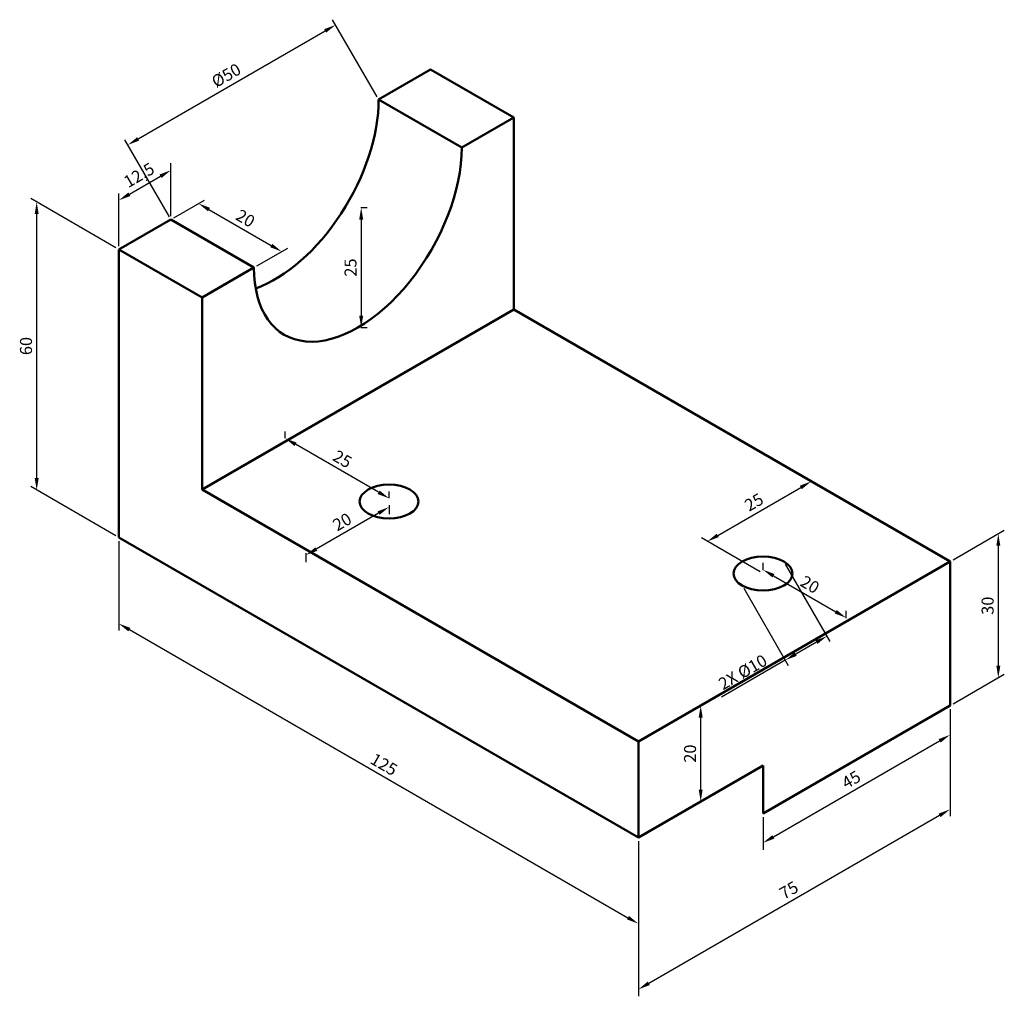
# Model space of a CAD drawing. Units: millimetres. Extents: x -63 to 142, y -21 to 183.
import ezdxf

# ---------------------------------------------------------------- set-up
doc = ezdxf.new("R2010")
doc.units = ezdxf.units.MM
for name, color, linetype, lineweight in [('M-CONS', 7, 'Continuous', 13), ('M-DIMS', 2, 'Continuous', 25), ('M-OUTL', 7, 'Continuous', 50)]:
    doc.layers.add(name, color=color, linetype=linetype, lineweight=lineweight)
doc.styles.get("Standard").update_dxf_attribs({"font": 'arial.ttf'})
doc.dimstyles.new('ISO-25', dxfattribs={"dimtxt": 2.5, "dimasz": 2.5, "dimexe": 1.25, "dimexo": 0.625, "dimtad": 1, "dimtxsty": 'Standard', "dimcen": 2.5, "dimadec": 0, "dimazin": 0, "dimtfac": 1, "dimtmove": 0, "dimatfit": 3, "dimfxl": 1, "dimarcsym": 0})

# ---------------------------------------------------------------- blocks, each defined once
blk = doc.blocks.new('*D1')
at = {"layer": 'Defpoints', "color": 0, "transparency": 16777216}
for p in [(91.92, 47.3), (78.93, 39.8), (91.92, 27.3)]:
    blk.add_point(p, dxfattribs=at)
at = {"layer": 'M-DIMS', "color": 0, "lineweight": -2, "transparency": 16777216}
for p, q in [((91.29, 46.94), (77.68, 39.08)), ((78.93, 22.3), (78.93, 37.3)), ((91.29, 26.94), (77.68, 19.08))]:
    blk.add_line(p, q, dxfattribs=at)
at = {"layer": 'M-DIMS', "color": 0, "transparency": 16777216}
for points in [[(78.51, 37.3), (79.34, 37.3), (78.93, 39.8)], [(78.51, 22.3), (79.34, 22.3), (78.93, 19.8)]]:
    blk.add_solid(points, dxfattribs=at)
at = {"layer": 'M-DIMS', "color": 0, "transparency": 16777216, "insert": (77.03, 29.8), "char_height": 2.5, "attachment_point": 5, "rotation": 90}
blk.add_mtext('20', dxfattribs=at)
blk = doc.blocks.new('*D2')
at = {"layer": 'Defpoints', "color": 0, "transparency": 16777216}
for p in [(130.89, 39.8), (130.89, 33.71), (91.92, 17.3)]:
    blk.add_point(p, dxfattribs=at)
at = {"layer": 'M-DIMS', "color": 0, "lineweight": -2, "transparency": 16777216}
for p, q in [((130.89, 39.08), (130.89, 32.26)), ((94.08, 12.46), (128.72, 32.46)), ((91.92, 16.58), (91.92, 9.76))]:
    blk.add_line(p, q, dxfattribs=at)
at = {"layer": 'M-DIMS', "color": 0, "transparency": 16777216}
for points in [[(128.52, 32.82), (128.93, 32.1), (130.89, 33.71)], [(93.87, 12.82), (94.29, 12.1), (91.92, 11.21)]]:
    blk.add_solid(points, dxfattribs=at)
at = {"layer": 'M-DIMS', "color": 0, "transparency": 16777216, "insert": (110.45, 24.1), "char_height": 2.5, "attachment_point": 5, "rotation": 30}
blk.add_mtext('45', dxfattribs=at)
blk = doc.blocks.new('*D3')
at = {"layer": 'Defpoints', "color": 0, "transparency": 16777216}
for p in [(130.89, 69.8), (140.95, 45.61), (130.89, 39.8)]:
    blk.add_point(p, dxfattribs=at)
at = {"layer": 'M-DIMS', "color": 0, "lineweight": -2, "transparency": 16777216}
for p, q in [((131.51, 70.16), (142.2, 76.33)), ((140.95, 73.11), (140.95, 48.11)), ((131.51, 40.16), (142.2, 46.33))]:
    blk.add_line(p, q, dxfattribs=at)
at = {"layer": 'M-DIMS', "color": 0, "transparency": 16777216}
for points in [[(140.54, 73.11), (141.37, 73.11), (140.95, 75.61)], [(140.54, 48.11), (141.37, 48.11), (140.95, 45.61)]]:
    blk.add_solid(points, dxfattribs=at)
at = {"layer": 'M-DIMS', "color": 0, "transparency": 16777216, "insert": (139.05, 60.61), "char_height": 2.5, "attachment_point": 5, "rotation": 90}
blk.add_mtext('30', dxfattribs=at)
blk = doc.blocks.new('*D4')
at = {"layer": 'Defpoints', "color": 0, "transparency": 16777216}
for p in [(130.89, 39.8), (65.94, 2.3), (65.94, -19.31)]:
    blk.add_point(p, dxfattribs=at)
at = {"layer": 'M-DIMS', "color": 0, "lineweight": -2, "transparency": 16777216}
for p, q in [((130.89, 39.08), (130.89, 16.75)), ((128.72, 16.94), (68.1, -18.06)), ((65.94, 1.58), (65.94, -20.75))]:
    blk.add_line(p, q, dxfattribs=at)
at = {"layer": 'M-DIMS', "color": 0, "transparency": 16777216}
for points in [[(128.52, 17.3), (128.93, 16.58), (130.89, 18.19)], [(67.89, -17.7), (68.31, -18.42), (65.94, -19.31)]]:
    blk.add_solid(points, dxfattribs=at)
at = {"layer": 'M-DIMS', "color": 0, "transparency": 16777216, "insert": (97.46, 1.08), "char_height": 2.5, "attachment_point": 5, "rotation": 30}
blk.add_mtext('75', dxfattribs=at)
blk = doc.blocks.new('*D5')
at = {"layer": 'Defpoints', "color": 0, "transparency": 16777216}
for p in [(101.96, 86.5), (113.57, 79.8), (91.92, 67.3)]:
    blk.add_point(p, dxfattribs=at)
at = {"layer": 'M-DIMS', "color": 0, "lineweight": -2, "transparency": 16777216}
for p, q in [((112.94, 80.16), (100.71, 87.22)), ((82.48, 75.25), (99.8, 85.25)), ((91.29, 67.66), (79.06, 74.72))]:
    blk.add_line(p, q, dxfattribs=at)
at = {"layer": 'M-DIMS', "color": 0, "transparency": 16777216}
for points in [[(99.59, 85.61), (100, 84.89), (101.96, 86.5)], [(82.27, 75.61), (82.68, 74.89), (80.31, 74)]]:
    blk.add_solid(points, dxfattribs=at)
at = {"layer": 'M-DIMS', "color": 0, "transparency": 16777216, "insert": (90.19, 81.9), "char_height": 2.5, "attachment_point": 5, "rotation": 30}
blk.add_mtext('25', dxfattribs=at)
blk = doc.blocks.new('*D6')
at = {"layer": 'Defpoints', "color": 0, "transparency": 16777216}
for p in [(91.92, 67.3), (109.24, 58.1), (109.24, 57.3)]:
    blk.add_point(p, dxfattribs=at)
at = {"layer": 'M-DIMS', "color": 0, "lineweight": -2, "transparency": 16777216}
for p, q in [((91.92, 68.02), (91.92, 69.54)), ((94.08, 66.85), (107.07, 59.35)), ((109.24, 58.02), (109.24, 59.54))]:
    blk.add_line(p, q, dxfattribs=at)
at = {"layer": 'M-DIMS', "color": 0, "transparency": 16777216}
for points in [[(94.29, 67.21), (93.87, 66.49), (91.92, 68.1)], [(107.28, 59.71), (106.86, 58.99), (109.24, 58.1)]]:
    blk.add_solid(points, dxfattribs=at)
at = {"layer": 'M-DIMS', "color": 0, "transparency": 16777216, "insert": (101.53, 64.74), "char_height": 2.5, "attachment_point": 5, "rotation": 330}
blk.add_mtext('20', dxfattribs=at)
blk = doc.blocks.new('*D7')
at = {"layer": 'Defpoints', "color": 0, "transparency": 16777216}
for p in [(13.98, 82.3), (-3.35, 72.3), (-3.35, 71.16)]:
    blk.add_point(p, dxfattribs=at)
at = {"layer": 'M-DIMS', "color": 0, "lineweight": -2, "transparency": 16777216}
for p, q in [((13.98, 81.58), (13.98, 79.71)), ((11.81, 79.91), (-1.18, 72.41)), ((-3.35, 71.58), (-3.35, 69.71))]:
    blk.add_line(p, q, dxfattribs=at)
at = {"layer": 'M-DIMS', "color": 0, "transparency": 16777216}
for points in [[(11.6, 80.27), (12.02, 79.55), (13.98, 81.16)], [(-1.39, 72.77), (-0.97, 72.05), (-3.35, 71.16)]]:
    blk.add_solid(points, dxfattribs=at)
at = {"layer": 'M-DIMS', "color": 0, "transparency": 16777216, "insert": (4.36, 77.8), "char_height": 2.5, "attachment_point": 5, "rotation": 30}
blk.add_mtext('20', dxfattribs=at)
blk = doc.blocks.new('*D8')
at = {"layer": 'Defpoints', "color": 0, "transparency": 16777216}
for p in [(-7.68, 95.48), (-7.68, 94.8), (13.98, 82.3)]:
    blk.add_point(p, dxfattribs=at)
at = {"layer": 'M-DIMS', "color": 0, "lineweight": -2, "transparency": 16777216}
for p, q in [((-7.68, 95.52), (-7.68, 96.93)), ((11.81, 84.23), (-5.51, 94.23)), ((13.98, 83.02), (13.98, 84.43))]:
    blk.add_line(p, q, dxfattribs=at)
at = {"layer": 'M-DIMS', "color": 0, "transparency": 16777216}
for points in [[(-5.3, 94.59), (-5.72, 93.87), (-7.68, 95.48)], [(12.02, 84.59), (11.6, 83.87), (13.98, 82.98)]]:
    blk.add_solid(points, dxfattribs=at)
at = {"layer": 'M-DIMS', "color": 0, "transparency": 16777216, "insert": (4.1, 90.88), "char_height": 2.5, "attachment_point": 5, "rotation": 330}
blk.add_mtext('25', dxfattribs=at)
blk = doc.blocks.new('*D9')
at = {"layer": 'Defpoints', "color": 0, "transparency": 16777216}
for p in [(-31.49, 151.32), (-31.49, 141.05), (-42.32, 134.8)]:
    blk.add_point(p, dxfattribs=at)
at = {"layer": 'M-DIMS', "color": 0, "lineweight": -2, "transparency": 16777216}
for p, q in [((-31.49, 141.77), (-31.49, 152.76)), ((-40.15, 146.32), (-33.66, 150.07)), ((-42.32, 135.52), (-42.32, 146.51))]:
    blk.add_line(p, q, dxfattribs=at)
at = {"layer": 'M-DIMS', "color": 0, "transparency": 16777216}
for points in [[(-33.86, 150.43), (-33.45, 149.7), (-31.49, 151.32)], [(-40.36, 146.68), (-39.94, 145.95), (-42.32, 145.07)]]:
    blk.add_solid(points, dxfattribs=at)
at = {"layer": 'M-DIMS', "color": 0, "transparency": 16777216, "insert": (-37.97, 150.03), "char_height": 2.5, "attachment_point": 5, "rotation": 30}
blk.add_mtext('12,5', dxfattribs=at)
blk = doc.blocks.new('*D10')
at = {"layer": 'Defpoints', "color": 0, "transparency": 16777216}
for p in [(-59.46, 144.7), (-42.32, 134.8), (-42.32, 74.8)]:
    blk.add_point(p, dxfattribs=at)
at = {"layer": 'M-DIMS', "color": 0, "lineweight": -2, "transparency": 16777216}
for p, q in [((-42.94, 135.16), (-60.71, 145.42)), ((-59.46, 87.2), (-59.46, 142.2)), ((-42.94, 75.16), (-60.71, 85.42))]:
    blk.add_line(p, q, dxfattribs=at)
at = {"layer": 'M-DIMS', "color": 0, "transparency": 16777216}
for points in [[(-59.88, 142.2), (-59.04, 142.2), (-59.46, 144.7)], [(-59.88, 87.2), (-59.04, 87.2), (-59.46, 84.7)]]:
    blk.add_solid(points, dxfattribs=at)
at = {"layer": 'M-DIMS', "color": 0, "transparency": 16777216, "insert": (-61.36, 114.7), "char_height": 2.5, "attachment_point": 5, "rotation": 90}
blk.add_mtext('60', dxfattribs=at)
blk = doc.blocks.new('*D11')
at = {"layer": 'Defpoints', "color": 0, "transparency": 16777216}
for p in [(-42.32, 74.8), (65.94, 12.3), (65.94, -5.63)]:
    blk.add_point(p, dxfattribs=at)
at = {"layer": 'M-DIMS', "color": 0, "lineweight": -2, "transparency": 16777216}
for p, q in [((-42.32, 74.08), (-42.32, 55.43)), ((-40.15, 55.62), (63.77, -4.38)), ((65.94, 11.58), (65.94, -7.07))]:
    blk.add_line(p, q, dxfattribs=at)
at = {"layer": 'M-DIMS', "color": 0, "transparency": 16777216}
for points in [[(-39.94, 55.98), (-40.36, 55.26), (-42.32, 56.87)], [(63.98, -4.02), (63.56, -4.74), (65.94, -5.63)]]:
    blk.add_solid(points, dxfattribs=at)
at = {"layer": 'M-DIMS', "color": 0, "transparency": 16777216, "insert": (12.76, 27.27), "char_height": 2.5, "attachment_point": 5, "rotation": 330}
blk.add_mtext('125', dxfattribs=at)
blk = doc.blocks.new('*D12')
at = {"layer": 'Defpoints', "color": 0, "transparency": 16777216}
for p in [(7.48, 143.55), (7.48, 118.55), (8.17, 118.55)]:
    blk.add_point(p, dxfattribs=at)
at = {"layer": 'M-DIMS', "color": 0, "lineweight": -2, "transparency": 16777216}
for p, q in [((8.11, 143.55), (9.42, 143.55)), ((8.17, 141.05), (8.17, 121.05)), ((8.11, 118.55), (9.42, 118.55))]:
    blk.add_line(p, q, dxfattribs=at)
at = {"layer": 'M-DIMS', "color": 0, "transparency": 16777216}
for points in [[(7.75, 141.05), (8.59, 141.05), (8.17, 143.55)], [(7.75, 121.05), (8.59, 121.05), (8.17, 118.55)]]:
    blk.add_solid(points, dxfattribs=at)
at = {"layer": 'M-DIMS', "color": 0, "transparency": 16777216, "insert": (6.27, 131.05), "char_height": 2.5, "attachment_point": 5, "rotation": 90}
blk.add_mtext('25', dxfattribs=at)
blk = doc.blocks.new('*D13')
at = {"layer": 'Defpoints', "color": 0, "transparency": 16777216}
for p in [(-31.49, 141.05), (-8.4, 134.38), (-14.17, 131.05)]:
    blk.add_point(p, dxfattribs=at)
at = {"layer": 'M-DIMS', "color": 0, "lineweight": -2, "transparency": 16777216}
for p, q in [((-30.87, 141.41), (-24.47, 145.11)), ((-23.55, 143.13), (-10.56, 135.63)), ((-13.55, 131.41), (-7.15, 135.11))]:
    blk.add_line(p, q, dxfattribs=at)
at = {"layer": 'M-DIMS', "color": 0, "transparency": 16777216}
for points in [[(-23.35, 143.49), (-23.76, 142.77), (-25.72, 144.38)], [(-10.36, 135.99), (-10.77, 135.27), (-8.4, 134.38)]]:
    blk.add_solid(points, dxfattribs=at)
at = {"layer": 'M-DIMS', "color": 0, "transparency": 16777216, "insert": (-16.11, 141.03), "char_height": 2.5, "attachment_point": 5, "rotation": 330}
blk.add_mtext('20', dxfattribs=at)
blk = doc.blocks.new('HOLE-D10-THRU-ISO')
blk.add_ellipse((6.12, 3.54), major_axis=(-6.12, 0), ratio=0.57735)
blk = doc.blocks.new('*D15')
at = {"layer": 'Defpoints', "color": 0, "transparency": 16777216}
for p in [(96.25, 69.8), (87.59, 64.8), (96.56, 49.26)]:
    blk.add_point(p, dxfattribs=at)
at = {"layer": 'M-DIMS', "color": 0, "lineweight": -2, "transparency": 16777216}
for p, q in [((96.56, 69.26), (105.85, 53.17)), ((87.9, 64.26), (97.19, 48.17)), ((103.06, 53.01), (98.73, 50.51)), ((96.56, 49.26), (83.29, 41.59))]:
    blk.add_line(p, q, dxfattribs=at)
at = {"layer": 'M-DIMS', "color": 0, "transparency": 16777216}
for points in [[(102.85, 53.37), (103.27, 52.65), (105.22, 54.26)], [(98.52, 50.87), (98.94, 50.15), (96.56, 49.26)]]:
    blk.add_solid(points, dxfattribs=at)
at = {"layer": 'M-DIMS', "color": 0, "transparency": 16777216, "insert": (87.86, 46.51), "char_height": 2.5, "attachment_point": 5, "rotation": 30}
blk.add_mtext('2X %%c10', dxfattribs=at)
blk = doc.blocks.new('*D16')
at = {"layer": 'Defpoints', "color": 0, "transparency": 16777216}
for p in [(2.84, 181.6), (11.81, 166.05), (-31.49, 141.05)]:
    blk.add_point(p, dxfattribs=at)
at = {"layer": 'M-DIMS', "color": 0, "lineweight": -2, "transparency": 16777216}
for p, q in [((11.5, 166.59), (2.21, 182.68)), ((-38.3, 157.85), (0.67, 180.35)), ((-31.8, 141.59), (-41.09, 157.68))]:
    blk.add_line(p, q, dxfattribs=at)
at = {"layer": 'M-DIMS', "color": 0, "transparency": 16777216}
for points in [[(0.46, 180.71), (0.88, 179.99), (2.84, 181.6)], [(-38.51, 158.21), (-38.09, 157.49), (-40.47, 156.6)]]:
    blk.add_solid(points, dxfattribs=at)
at = {"layer": 'M-DIMS', "color": 0, "transparency": 16777216, "insert": (-19.8, 170.8), "char_height": 2.5, "attachment_point": 5, "rotation": 30}
blk.add_mtext('%%c50', dxfattribs=at)

msp = doc.modelspace()

# ---------------------------------------------------------------- linework, layer by layer
at = {"layer": 'M-CONS'}
msp.add_line((130.889, 69.802), (113.568, 79.802), dxfattribs=at)
at = {"layer": 'M-OUTL'}
for p, q in [((11.81, 166.052), (22.635, 172.302)), ((22.635, 172.302), (39.956, 162.302)), ((29.131, 156.052), (11.81, 166.052)), ((39.956, 162.302), (29.131, 156.052)), ((39.956, 122.302), (39.956, 162.302)), ((-42.316, 134.802), (-31.491, 141.052)), ((-31.491, 141.052), (-14.171, 131.052)), ((-42.316, 74.802), (-42.316, 134.802)), ((-42.316, 134.802), (-24.996, 124.802)), ((-14.171, 131.052), (-24.996, 124.802)), ((-24.996, 124.802), (-24.996, 84.802)), ((-24.996, 84.802), (39.956, 122.302)), ((39.956, 122.302), (130.889, 69.802)), ((-24.996, 84.802), (65.937, 32.302)), ((-42.316, 74.802), (65.937, 12.302)), ((130.889, 69.802), (65.937, 32.302)), ((130.889, 39.802), (130.889, 69.802)), ((91.918, 17.302), (130.889, 39.802)), ((65.937, 32.302), (65.937, 12.302)), ((65.937, 12.302), (91.918, 27.302)), ((91.918, 27.302), (91.918, 17.302))]:
    msp.add_line(p, q, dxfattribs=at)
for centre, start_param in [((-9.84, 153.552), 6.8844495), ((7.48, 143.552), 5.4977871)]:
    msp.add_ellipse(centre, major_axis=(-15.309, -26.517), ratio=0.5773503, start_param=start_param, end_param=8.6393798, dxfattribs=at)

# ---------------------------------------------------------------- block references
for p in [(7.852, 78.766), (85.794, 63.766)]:
    msp.add_blockref('HOLE-D10-THRU-ISO', p, dxfattribs=at)

# ---------------------------------------------------------------- dimensions: what is measured, and where the dimension line sits
at = {"layer": 'M-DIMS'}
for base, p1, p2, angle, text, picture, middle in [((2.835, 181.597), (-31.491, 141.052), (11.81, 166.052), 30, '%%c<>', '*D16', (-19.801, 170.804)), ((96.562, 49.256), (96.248, 69.802), (87.587, 64.802), 210, '2X %%c<>', '*D15', (87.859, 46.508))]:
    dim = msp.add_linear_dim(base=base, p1=p1, p2=p2, angle=angle, text=text, dimstyle='ISO-25', override={"dimdec": 0, "dimlfac": 1, "dimrnd": 0, "dimzin": 0, "dimdsep": 46, "dimlunit": 2}, dxfattribs=at)
    dim.commit()
    dim.dimension.update_dxf_attribs({"geometry": picture, "text_midpoint": middle})
for p1, p2, distance, picture, middle in [((-42.316, 134.802), (-31.491, 141.052), 8.889, '*D9', (-37.967, 150.033)), ((-31.491, 141.052), (-14.171, 131.052), 5.772, '*D13', (-16.108, 141.031)), ((13.975, 82.302), (-7.675, 94.802), -0.591, '*D8', (4.101, 90.88)), ((91.918, 67.302), (113.568, 79.802), 11.607, '*D5', (90.185, 81.9)), ((13.975, 82.302), (-3.345, 72.302), 0.991, '*D7', (4.364, 77.804)), ((-42.316, 74.802), (65.937, 12.302), -15.527, '*D11', (12.761, 27.269)), ((91.918, 67.302), (109.238, 57.302), 0.689, '*D6', (101.529, 64.744)), ((130.889, 39.802), (65.937, 2.302), 18.717, '*D4', (97.465, 1.081)), ((91.918, 17.302), (130.889, 39.802), -5.279, '*D2', (110.455, 24.098))]:
    dim = msp.add_aligned_dim(p1=p1, p2=p2, distance=distance, dimstyle='ISO-25', override={"dimclrd": 0, "dimclre": 0, "dimclrt": 0}, dxfattribs=at)
    dim.commit()
    dim.dimension.update_dxf_attribs({"geometry": picture, "text_midpoint": middle})
for base, p1, p2, picture, middle in [((-59.459, 144.699), (-42.316, 74.802), (-42.316, 134.802), '*D10', (-61.36, 114.699)), ((8.171, 118.552), (7.48, 143.552), (7.48, 118.552), '*D12', (6.27, 131.052)), ((140.953, 45.612), (130.889, 69.802), (130.889, 39.802), '*D3', (139.05, 60.612)), ((78.927, 39.802), (91.918, 27.302), (91.918, 47.302), '*D1', (77.026, 29.802))]:
    dim = msp.add_linear_dim(base=base, p1=p1, p2=p2, angle=90, dimstyle='ISO-25', override={"dimclrd": 0, "dimclre": 0, "dimclrt": 0}, dxfattribs=at)
    dim.commit()
    dim.dimension.update_dxf_attribs({"geometry": picture, "text_midpoint": middle})

doc.saveas('drawing.dxf')
